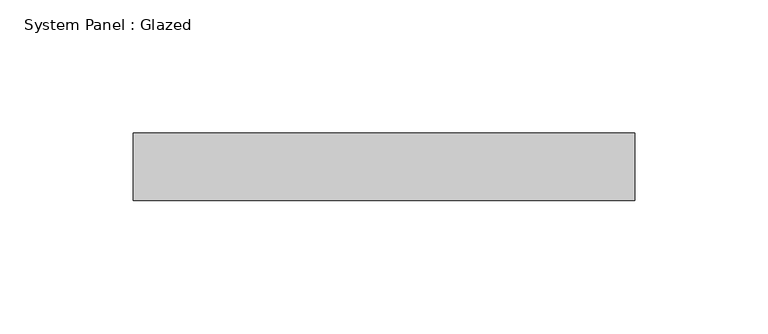
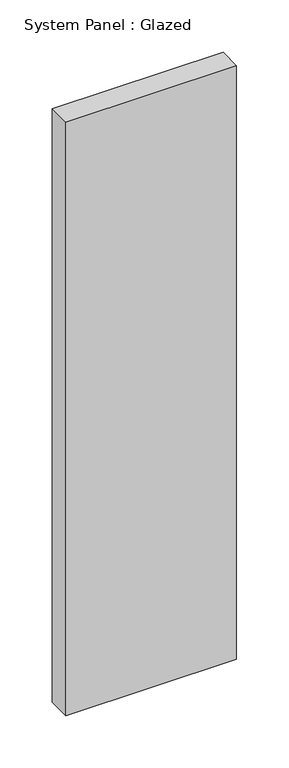
"""IFC4 building model written with IfcOpenShell, lengths in millimetres: plate geometry, System Panel : Glazed."""

from ifc_helpers import new_model, si_unit, origin, origin_with_axes, place, context, project, spatial, polyline, outline, extrude, source, transform, mapped, element, save


def system_panel_glazed_71f4521f(model_context):
    return source(origin(), model_context, "Body", "SweptSolid", [
        extrude(outline(polyline([(94.1916667, 19.05), (-94.1916667, 19.05), (-94.1916667, 44.45), (94.1916667, 44.45), (94.1916667, 19.05)])), origin_with_axes(), (0.0, 0.0, 1.0), 692.15),
    ])


if __name__ == "__main__":
    model = new_model("IFC4")
    model_context = context("Model", 3, world=origin())
    ifc_project = project(units=[si_unit("LENGTHUNIT", "METRE", prefix="MILLI")], contexts=[model_context])
    site = spatial("IfcSite", under=ifc_project)
    building = spatial("IfcBuilding", under=site)
    placement = place(None, origin())
    system_panel_glazed_shape = system_panel_glazed_71f4521f(model_context)
    element("IfcPlate", 1, ObjectType="System Panel : Glazed", at=placement, inside=building, context=model_context, shape_type="MappedRepresentation", body=[
        mapped(system_panel_glazed_shape, transform((0.0, 0.0, 0.0), x_axis=(1.0, 0.0, 0.0), y_axis=(0.0, 1.0, 0.0), z_axis=(0.0, 0.0, 1.0))),
    ])
    save(model, "model.ifc")

# Revit data of these elements
# Type "System Panel : Glazed"
#   Construction Type Id = "GSP4R"
#   Analytic Construction = "1/8 in Pilkington single glazing"
#   Visual Light Transmittance = 0.9
#   Solar Heat Gain Coefficient = 0.86
#   Heat Transfer Coefficient (U) = 1.18115 BTU/(h·ft²·°F)
#   Define Thermal Properties by = 1
# Element 1 (IfcPlate, "System Panel : Glazed")
#   Materials on its faces: "Glass"
# Materials
#   "Glass": class "Glass", colour RGB 0 128 192, transparency 0.75, Description = "Soda Lime Glass", Cost = 0
